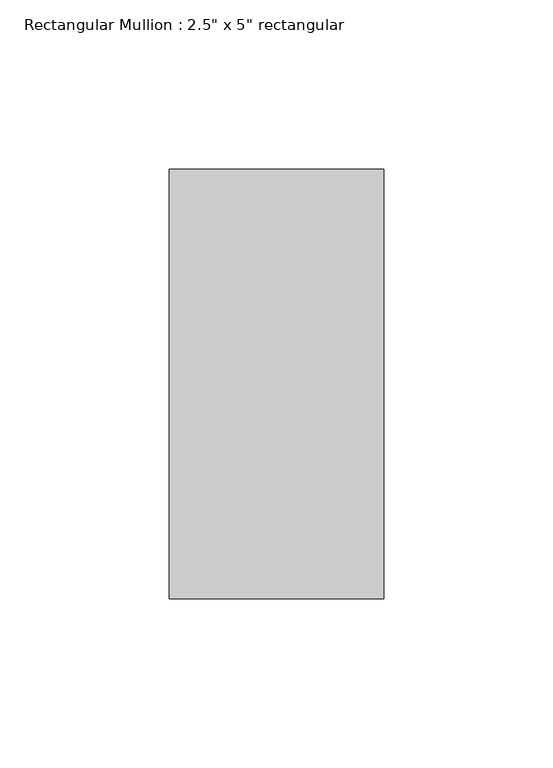
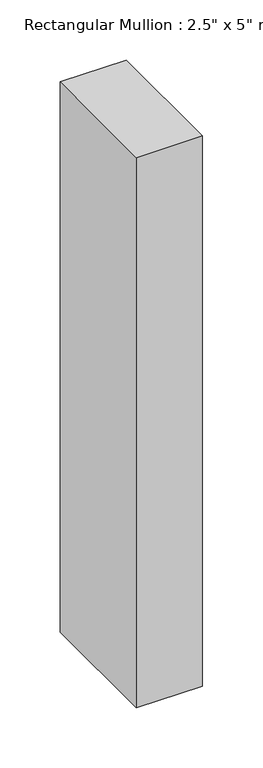
"""IFC4 building model written with IfcOpenShell, lengths in millimetres: member geometry."""

from ifc_helpers import new_model, si_unit, frame, origin, place, context, project, spatial, polyline, outline, extrude, source, transform, mapped, element, save


def member_50cacee6(model_context):
    return source(origin(), model_context, "Body", "SweptSolid", [
        extrude(outline(polyline([(0.0, 63.5), (0.0, -63.5), (-63.5, -63.5), (-63.5, 63.5), (0.0, 63.5)])), frame((0.0, 0.0, -558.8), z_axis=(0.0, 0.0, 1.0), x_axis=(1.0, 0.0, 0.0)), (0.0, 0.0, 1.0), 558.8),
    ])


if __name__ == "__main__":
    model = new_model("IFC4")
    model_context = context("Model", 3, world=origin())
    ifc_project = project(units=[si_unit("LENGTHUNIT", "METRE", prefix="MILLI")], contexts=[model_context])
    site = spatial("IfcSite", under=ifc_project)
    building = spatial("IfcBuilding", under=site)
    placement = place(None, origin())
    member_shape = member_50cacee6(model_context)
    element("IfcMember", 1, ObjectType="Rectangular Mullion : 2.5\" x 5\" rectangular", at=placement, inside=building, context=model_context, shape_type="MappedRepresentation", body=[
        mapped(member_shape, transform((0.0, 0.0, 0.0), x_axis=(1.0, 0.0, 0.0), y_axis=(0.0, 1.0, 0.0), z_axis=(0.0, 0.0, 1.0))),
    ])
    save(model, "model.ifc")

# Revit data of these elements
# Type "Rectangular Mullion : 2.5\" x 5\" rectangular"
#   built-in parameter 1007304 = 0.416667 (stored number, unit not read)
#   built-in parameter 1007301 = 0.104167 (stored number, unit not read)
#   built-in parameter 1007300 = 0.104167 (stored number, unit not read)
# Element 1 (IfcMember, "Rectangular Mullion : 2.5\" x 5\" rectangular")
#   Materials on its faces: "Rectangle 1 sq"
# Materials
#   "Rectangle 1 sq": class "Generic", colour RGB 120 120 120, transparency 0, Cost = 0
